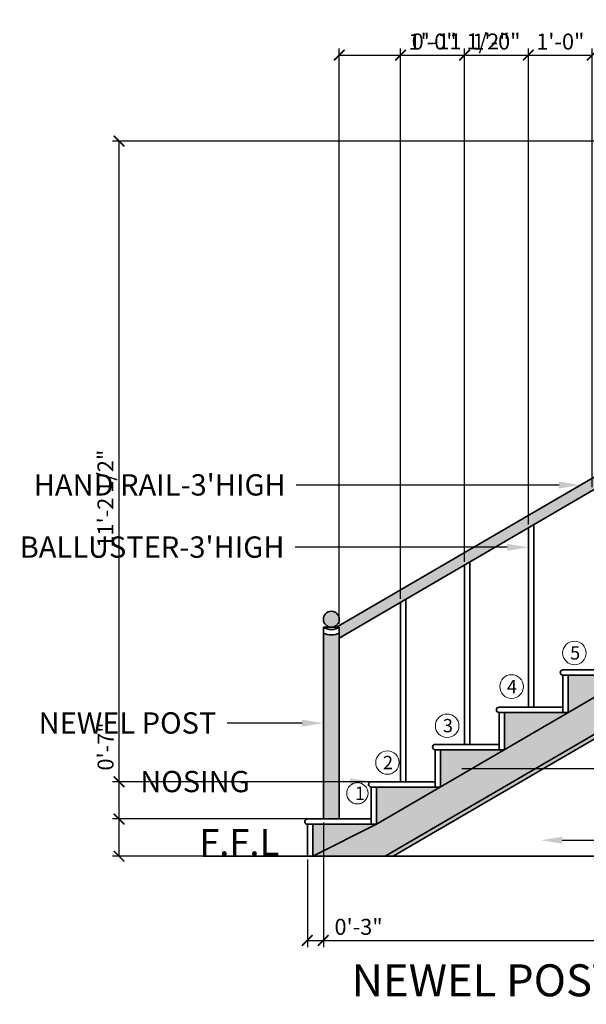
# Model space of a CAD drawing. Units: inches. Extents: x 2205 to 2524, y 4609 to 4803.
# Tile 1 of 5: x 2205 to 2311, y 4609 to 4794. Entities that reach past the tile are written whole.
import ezdxf
from ezdxf import colors
from ezdxf.entities.mleader import LeaderData, LeaderLine
from ezdxf.math import Vec2, Vec3

# ---------------------------------------------------------------- set-up
doc = ezdxf.new("R2010")
doc.units = ezdxf.units.IN
for name, color, linetype, lineweight in [('A-ANNO-DIMS', 2, 'Continuous', 18), ('A-ANNO-SYMB', 3, 'Continuous', 18), ('A-ANNO-TEXT', 7, 'Continuous', 18), ('A-FLOR-STRS', 7, 'Continuous', 35), ('A-SECT', 7, 'Continuous', 25), ('A-SECT-PATT', 252, 'Continuous', 13)]:
    doc.layers.add(name, color=color, linetype=linetype, lineweight=lineweight)
doc.styles.get("Standard").update_dxf_attribs({"font": 'arial.ttf'})
doc.dimstyles.new('ISO-25', dxfattribs={"dimtxt": 3, "dimasz": 2, "dimexe": 1.25, "dimexo": 0.625, "dimtad": 1, "dimdec": 1, "dimlunit": 3, "dimtxsty": 'Standard', "dimblk": 'ARCHTICK', "dimcen": 2.5, "dimclrd": 5, "dimclre": 2, "dimclrt": 6, "dimadec": 0, "dimazin": 0, "dimtfac": 1, "dimtdec": 1, "dimtmove": 0, "dimatfit": 3, "dimfxl": 1, "dimarcsym": 0})

# ---------------------------------------------------------------- blocks, each defined once
blk = doc.blocks.new('STAIR-STEP')
for p, q in [((2282.7, 4650.98), (2270.7, 4650.98)), ((2283.7, 4649.98), (2270.7, 4649.98)), ((2270.7, 4649.98), (2270.7, 4642.98)), ((2271.7, 4649.98), (2271.7, 4642.98))]:
    blk.add_line(p, q)
blk.add_arc((2270.7, 4650.48), 0.5, 90, 270)
blk = doc.blocks.new('NEWEL-POST')
for p, q in [((2261.7, 4679.98), (2261.7, 4643.98)), ((2261.71, 4679.98), (2261.7, 4679.98)), ((2261.71, 4679.98), (2264.69, 4679.98)), ((2264.7, 4679.98), (2264.69, 4679.98)), ((2264.7, 4679.98), (2264.7, 4643.98))]:
    blk.add_line(p, q)
blk.add_circle((2263.2, 4681.48), 1.5)
for radius, start, end in [(2.78, 237.6128, 302.3872), (3.78, 246.6124, 293.3876)]:
    blk.add_arc((2263.2, 4682.33), radius, start, end)
blk = doc.blocks.new('BALUSTER')
for p, q in [((2276.2, 4684.66), (2276.2, 4650.98)), ((2277.2, 4685.25), (2277.2, 4650.98))]:
    blk.add_line(p, q)
blk = doc.blocks.new('_ArchTick')
at = {"color": 0, "linetype": 'ByBlock', "const_width": 0.15}
blk.add_lwpolyline([(-0.5, -0.5), (0.5, 0.5)], dxfattribs=at)
blk = doc.blocks.new('*D15')
at = {"layer": 'A-ANNO-DIMS', "color": 2, "lineweight": -2, "transparency": 16777216}
for p, q in [((2258.7, 4636.35), (2258.7, 4619.93)), ((2429.2, 4636.35), (2429.2, 4619.93))]:
    blk.add_line(p, q, dxfattribs=at)
at = {"layer": 'A-ANNO-DIMS', "color": 5, "lineweight": -2, "transparency": 16777216}
blk.add_line((2258.7, 4621.18), (2429.2, 4621.18), dxfattribs=at)
at = {"layer": 'DEFPOINTS', "color": 0, "transparency": 16777216}
for p in [(2258.7, 4636.98), (2429.2, 4636.98), (2429.2, 4621.18)]:
    blk.add_point(p, dxfattribs=at)
at = {"layer": 'A-ANNO-DIMS', "color": 5, "lineweight": -2, "transparency": 16777216, "xscale": 2, "yscale": 2, "zscale": 2, "rotation": 180}
blk.add_blockref('_ArchTick', (2258.7, 4621.18), dxfattribs=at)
at = {"layer": 'A-ANNO-DIMS', "color": 5, "lineweight": -2, "transparency": 16777216, "xscale": 2, "yscale": 2, "zscale": 2}
blk.add_blockref('_ArchTick', (2429.2, 4621.18), dxfattribs=at)
at = {"layer": 'A-ANNO-DIMS', "color": 6, "transparency": 16777216, "insert": (2343.95, 4623.36), "char_height": 3, "attachment_point": 5}
blk.add_mtext('14\'-2 1/2"', dxfattribs=at)
blk = doc.blocks.new('*D16')
at = {"layer": 'A-ANNO-DIMS', "color": 2, "lineweight": -2, "transparency": 16777216}
for p, q in [((2428.57, 4771.26), (2222.09, 4771.26)), ((2428.57, 4636.98), (2222.09, 4636.98))]:
    blk.add_line(p, q, dxfattribs=at)
at = {"layer": 'A-ANNO-DIMS', "color": 5, "lineweight": -2, "transparency": 16777216}
blk.add_line((2223.34, 4636.98), (2223.34, 4771.26), dxfattribs=at)
at = {"layer": 'DEFPOINTS', "color": 0, "transparency": 16777216}
for p in [(2223.34, 4771.26), (2429.2, 4771.26), (2429.2, 4636.98)]:
    blk.add_point(p, dxfattribs=at)
at = {"layer": 'A-ANNO-DIMS', "color": 5, "lineweight": -2, "transparency": 16777216, "xscale": 2, "yscale": 2, "zscale": 2}
for p, rotation in [((2223.34, 4771.26), 90), ((2223.34, 4636.98), 270)]:
    blk.add_blockref('_ArchTick', p, dxfattribs=dict(at, rotation=rotation))
at = {"layer": 'A-ANNO-DIMS', "color": 6, "transparency": 16777216, "insert": (2221.17, 4704.12), "char_height": 3, "attachment_point": 5, "rotation": 90}
blk.add_mtext('11\'-2 1/2"', dxfattribs=at)
blk = doc.blocks.new('*D18')
at = {"layer": 'A-ANNO-DIMS', "color": 5, "lineweight": -2, "transparency": 16777216}
for p, q in [((2223.34, 4650.98), (2223.34, 4662.2)), ((2223.34, 4643.98), (2223.34, 4650.98))]:
    blk.add_line(p, q, dxfattribs=at)
at = {"layer": 'A-ANNO-DIMS', "color": 2, "lineweight": -2, "transparency": 16777216}
for p, q in [((2275.57, 4650.98), (2222.09, 4650.98)), ((2264.07, 4643.98), (2222.09, 4643.98))]:
    blk.add_line(p, q, dxfattribs=at)
at = {"layer": 'DEFPOINTS', "color": 0, "transparency": 16777216}
for p in [(2223.34, 4650.98), (2276.2, 4650.98), (2264.7, 4643.98)]:
    blk.add_point(p, dxfattribs=at)
at = {"layer": 'A-ANNO-DIMS', "color": 5, "lineweight": -2, "transparency": 16777216, "xscale": 2, "yscale": 2, "zscale": 2}
for p, rotation in [((2223.34, 4650.98), 90), ((2223.34, 4643.98), 270)]:
    blk.add_blockref('_ArchTick', p, dxfattribs=dict(at, rotation=rotation))
at = {"layer": 'A-ANNO-DIMS', "color": 6, "transparency": 16777216, "insert": (2221.19, 4657.59), "char_height": 3, "attachment_point": 5, "rotation": 90}
blk.add_mtext('0\'-7"', dxfattribs=at)
blk = doc.blocks.new('*D24')
at = {"layer": 'A-ANNO-DIMS', "color": 2, "lineweight": -2, "transparency": 16777216}
for p, q in [((2261.7, 4643.35), (2261.7, 4619.93)), ((2258.7, 4636.35), (2258.7, 4619.93))]:
    blk.add_line(p, q, dxfattribs=at)
at = {"layer": 'A-ANNO-DIMS', "color": 5, "lineweight": -2, "transparency": 16777216}
for p, q in [((2258.7, 4621.18), (2261.7, 4621.18)), ((2261.7, 4621.18), (2272.92, 4621.18))]:
    blk.add_line(p, q, dxfattribs=at)
at = {"layer": 'DEFPOINTS', "color": 0, "transparency": 16777216}
for p in [(2261.7, 4643.98), (2258.7, 4636.98), (2261.7, 4621.18)]:
    blk.add_point(p, dxfattribs=at)
at = {"layer": 'A-ANNO-DIMS', "color": 5, "lineweight": -2, "transparency": 16777216, "xscale": 2, "yscale": 2, "zscale": 2, "rotation": 180}
blk.add_blockref('_ArchTick', (2258.7, 4621.18), dxfattribs=at)
at = {"layer": 'A-ANNO-DIMS', "color": 5, "lineweight": -2, "transparency": 16777216, "xscale": 2, "yscale": 2, "zscale": 2}
blk.add_blockref('_ArchTick', (2261.7, 4621.18), dxfattribs=at)
at = {"layer": 'A-ANNO-DIMS', "color": 6, "transparency": 16777216, "insert": (2268.31, 4623.34), "char_height": 3, "attachment_point": 5}
blk.add_mtext('0\'-3"', dxfattribs=at)
blk = doc.blocks.new('*D26')
at = {"layer": 'A-ANNO-DIMS', "color": 2, "lineweight": -2, "transparency": 16777216}
for p, q in [((2264.7, 4680.6), (2264.7, 4788.66)), ((2276.2, 4685.29), (2276.2, 4788.66))]:
    blk.add_line(p, q, dxfattribs=at)
at = {"layer": 'A-ANNO-DIMS', "color": 5, "lineweight": -2, "transparency": 16777216}
for p, q in [((2264.7, 4787.41), (2276.2, 4787.41)), ((2276.2, 4787.41), (2296.74, 4787.41))]:
    blk.add_line(p, q, dxfattribs=at)
at = {"layer": 'DEFPOINTS', "color": 0, "transparency": 16777216}
for p in [(2276.2, 4787.41), (2276.2, 4684.66), (2264.7, 4679.98)]:
    blk.add_point(p, dxfattribs=at)
at = {"layer": 'A-ANNO-DIMS', "color": 5, "lineweight": -2, "transparency": 16777216, "xscale": 2, "yscale": 2, "zscale": 2, "rotation": 180}
blk.add_blockref('_ArchTick', (2264.7, 4787.41), dxfattribs=at)
at = {"layer": 'A-ANNO-DIMS', "color": 5, "lineweight": -2, "transparency": 16777216, "xscale": 2, "yscale": 2, "zscale": 2}
blk.add_blockref('_ArchTick', (2276.2, 4787.41), dxfattribs=at)
at = {"layer": 'A-ANNO-DIMS', "color": 6, "transparency": 16777216, "insert": (2287.47, 4789.58), "char_height": 3, "attachment_point": 5}
blk.add_mtext('0\'-11 1/2"', dxfattribs=at)
blk = doc.blocks.new('*D27')
at = {"layer": 'A-ANNO-DIMS', "color": 2, "lineweight": -2, "transparency": 16777216}
for p, q in [((2276.2, 4685.29), (2276.2, 4788.66)), ((2288.2, 4692.29), (2288.2, 4788.66))]:
    blk.add_line(p, q, dxfattribs=at)
at = {"layer": 'A-ANNO-DIMS', "color": 5, "lineweight": -2, "transparency": 16777216}
blk.add_line((2276.2, 4787.41), (2288.2, 4787.41), dxfattribs=at)
at = {"layer": 'DEFPOINTS', "color": 0, "transparency": 16777216}
for p in [(2288.2, 4787.41), (2288.2, 4691.66), (2276.2, 4684.66)]:
    blk.add_point(p, dxfattribs=at)
at = {"layer": 'A-ANNO-DIMS', "color": 5, "lineweight": -2, "transparency": 16777216, "xscale": 2, "yscale": 2, "zscale": 2, "rotation": 180}
blk.add_blockref('_ArchTick', (2276.2, 4787.41), dxfattribs=at)
at = {"layer": 'A-ANNO-DIMS', "color": 5, "lineweight": -2, "transparency": 16777216, "xscale": 2, "yscale": 2, "zscale": 2}
blk.add_blockref('_ArchTick', (2288.2, 4787.41), dxfattribs=at)
at = {"layer": 'A-ANNO-DIMS', "color": 6, "transparency": 16777216, "insert": (2282.2, 4789.56), "char_height": 3, "attachment_point": 5}
blk.add_mtext('1\'-0"', dxfattribs=at)
blk = doc.blocks.new('*D28')
at = {"layer": 'A-ANNO-DIMS', "color": 2, "lineweight": -2, "transparency": 16777216}
for p, q in [((2288.2, 4692.29), (2288.2, 4788.66)), ((2300.2, 4699.29), (2300.2, 4788.66))]:
    blk.add_line(p, q, dxfattribs=at)
at = {"layer": 'A-ANNO-DIMS', "color": 5, "lineweight": -2, "transparency": 16777216}
blk.add_line((2288.2, 4787.41), (2300.2, 4787.41), dxfattribs=at)
at = {"layer": 'DEFPOINTS', "color": 0, "transparency": 16777216}
for p in [(2300.2, 4787.41), (2300.2, 4698.66), (2288.2, 4691.66)]:
    blk.add_point(p, dxfattribs=at)
at = {"layer": 'A-ANNO-DIMS', "color": 5, "lineweight": -2, "transparency": 16777216, "xscale": 2, "yscale": 2, "zscale": 2, "rotation": 180}
blk.add_blockref('_ArchTick', (2288.2, 4787.41), dxfattribs=at)
at = {"layer": 'A-ANNO-DIMS', "color": 5, "lineweight": -2, "transparency": 16777216, "xscale": 2, "yscale": 2, "zscale": 2}
blk.add_blockref('_ArchTick', (2300.2, 4787.41), dxfattribs=at)
at = {"layer": 'A-ANNO-DIMS', "color": 6, "transparency": 16777216, "insert": (2294.2, 4789.56), "char_height": 3, "attachment_point": 5}
blk.add_mtext('1\'-0"', dxfattribs=at)
blk = doc.blocks.new('*D29')
at = {"layer": 'A-ANNO-DIMS', "color": 2, "lineweight": -2, "transparency": 16777216}
for p, q in [((2300.2, 4699.29), (2300.2, 4788.66)), ((2312.2, 4706.29), (2312.2, 4788.66))]:
    blk.add_line(p, q, dxfattribs=at)
at = {"layer": 'A-ANNO-DIMS', "color": 5, "lineweight": -2, "transparency": 16777216}
blk.add_line((2300.2, 4787.41), (2312.2, 4787.41), dxfattribs=at)
at = {"layer": 'DEFPOINTS', "color": 0, "transparency": 16777216}
for p in [(2312.2, 4787.41), (2312.2, 4705.66), (2300.2, 4698.66)]:
    blk.add_point(p, dxfattribs=at)
at = {"layer": 'A-ANNO-DIMS', "color": 5, "lineweight": -2, "transparency": 16777216, "xscale": 2, "yscale": 2, "zscale": 2, "rotation": 180}
blk.add_blockref('_ArchTick', (2300.2, 4787.41), dxfattribs=at)
at = {"layer": 'A-ANNO-DIMS', "color": 5, "lineweight": -2, "transparency": 16777216, "xscale": 2, "yscale": 2, "zscale": 2}
blk.add_blockref('_ArchTick', (2312.2, 4787.41), dxfattribs=at)
at = {"layer": 'A-ANNO-DIMS', "color": 6, "transparency": 16777216, "insert": (2306.2, 4789.56), "char_height": 3, "attachment_point": 5}
blk.add_mtext('1\'-0"', dxfattribs=at)

msp = doc.modelspace()

# ---------------------------------------------------------------- hatches: boundary and pattern name
at = {"layer": 'A-SECT-PATT'}
h = msp.add_hatch(dxfattribs=at)
h.set_pattern_fill('AR-CONC', color=256, scale=0.04)
h.paths.add_polyline_path([(2393.32, 4706.98), (2419.45, 4706.98), (2425.45, 4706.98), (2425.45, 4712.98), (2419.45, 4712.98), (2379.7, 4712.98), (2379.7, 4705.98), (2271.7, 4642.98), (2259.7, 4636.98), (2273.32, 4636.98)])
h.paths.add_polyline_path([(2343.7, 4684.98), (2331.7, 4684.98), (2331.7, 4677.98)], flags=16)
h.paths.add_polyline_path([(2331.7, 4677.98), (2319.7, 4677.98), (2319.7, 4670.98)], flags=16)
h.paths.add_polyline_path([(2319.7, 4670.98), (2307.7, 4670.98), (2307.7, 4663.98)], flags=16)
h.paths.add_polyline_path([(2307.7, 4663.98), (2295.7, 4663.98), (2295.7, 4656.98)], flags=16)
h.paths.add_polyline_path([(2295.7, 4656.98), (2283.7, 4656.98), (2283.7, 4649.98)], flags=16)
h.paths.add_polyline_path([(2283.7, 4649.98), (2271.7, 4649.98), (2271.7, 4642.98)], flags=17)
h.paths.add_polyline_path([(2271.7, 4642.98), (2259.7, 4642.98), (2259.7, 4636.98)], flags=17)
h.paths.add_polyline_path([(2379.7, 4705.98), (2367.7, 4705.98), (2367.7, 4698.98)], flags=16)
h.paths.add_polyline_path([(2367.7, 4698.98), (2355.7, 4698.98), (2355.7, 4691.98)], flags=16)
h.paths.add_polyline_path([(2419.45, 4706.98), (2393.32, 4706.98), (2273.32, 4636.98), (2274.81, 4636.98), (2393.52, 4706.23), (2419.45, 4706.23)], flags=17)
h.paths.add_polyline_path([(2419.45, 4706.23), (2418.7, 4706.23), (2418.7, 4636.98), (2419.45, 4636.98)], flags=16)
h.paths.add_polyline_path([(2429.2, 4771.26), (2428.45, 4771.26), (2428.45, 4636.98), (2429.2, 4636.98)])
h.paths.add_polyline_path([(2419.45, 4771.26), (2418.7, 4771.26), (2418.7, 4713.98), (2419.45, 4713.98)])
h = msp.add_hatch(color=256, dxfattribs=at)
h.dxf.hatch_style = 1
h.paths.add_polyline_path([(2264.7, 4678.86, -0.206977), (2261.7, 4678.86), (2261.7, 4643.98), (2264.7, 4643.98)])
h.paths.add_polyline_path([(2261.7, 4681.48, 1), (2264.7, 4681.48, 1)])
h.paths.add_polyline_path([(2382.06, 4746.42), (2382.06, 4748.73), (2264.2, 4679.98), (2264.69, 4679.98), (2264.7, 4679.98), (2264.7, 4677.96)])
h.paths.add_polyline_path([(2418.7, 4748.73), (2385.06, 4748.73), (2385.06, 4746.73), (2418.7, 4746.73)])
h.paths.add_polyline_path([(2385.06, 4748.86, -0.206977), (2382.06, 4748.86), (2382.06, 4713.98), (2385.06, 4713.98)])
h.paths.add_polyline_path([(2382.06, 4751.48, 1), (2385.06, 4751.48, 1)])

# ---------------------------------------------------------------- linework, layer by layer
at = {"layer": 'A-ANNO-SYMB'}
for centre, radius in [((2308.85, 4675.15), 2.21), ((2297.05, 4668.85), 2.22), ((2284.95, 4661.48), 2.21), ((2273.73, 4654.57), 2.2), ((2268.09, 4648.81), 2)]:
    msp.add_circle(centre, radius, dxfattribs=at)
at = {"layer": 'A-FLOR-STRS'}
for p, q in [((2264.2, 4679.98), (2382.06, 4748.73)), ((2264.7, 4677.96), (2382.06, 4746.42)), ((2273.32, 4636.98), (2393.32, 4706.98)), ((2271.7, 4642.98), (2379.7, 4705.98)), ((2274.81, 4636.98), (2393.52, 4706.23)), ((2270.7, 4643.98), (2258.7, 4643.98)), ((2271.7, 4642.98), (2258.7, 4642.98)), ((2258.7, 4642.98), (2258.7, 4636.98)), ((2259.7, 4642.98), (2259.7, 4636.98)), ((2271.7, 4642.98), (2259.7, 4636.98))]:
    msp.add_line(p, q, dxfattribs=at)
msp.add_arc((2258.7, 4643.48), 0.5, 90, 270, dxfattribs=at)
at = {"layer": 'A-SECT'}
msp.add_line((2239.14, 4636.98), (2429.2, 4636.98), dxfattribs=at)

# ---------------------------------------------------------------- block references
at = {"layer": 'A-FLOR-STRS'}
for name, p in [('BALUSTER', (24, 14)), ('BALUSTER', (12, 7)), ('BALUSTER', (0, 0)), ('NEWEL-POST', (0, 0)), ('STAIR-STEP', (36, 21)), ('STAIR-STEP', (24, 14)), ('STAIR-STEP', (12, 7)), ('STAIR-STEP', (0, 0))]:
    msp.add_blockref(name, p, dxfattribs=at)

# ---------------------------------------------------------------- texts
at = {"layer": 'A-ANNO-TEXT', "attachment_point": 1}
for s, width, heights, insert, char_height in [('5', 3.6522, [0], (2308.03, 4676.42), 2.5), ('4', 3.6522, [0], (2296.18, 4670.1), 2.5), ('3', 3.6522, [0], (2284.14, 4662.76), 2.5), ('2', 3.6522, [0], (2272.9, 4655.83), 2.5), ('1', 3.6522, [0], (2267.63, 4650.06), 2.5), ('F.F.L', 13.5213, [3.64], (2238.39, 4642.09), 5), ('{\\fArial|b1|i0|c0|p34;NEWEL POST QUATER TURN STAIR}', 215.8477, [0], (2266.99, 4616.69), 6)]:
    msp.add_mtext_dynamic_manual_height_columns(s, width=width, gutter_width=12.5, heights=heights, dxfattribs=dict(at, insert=insert, char_height=char_height))

# ---------------------------------------------------------------- dimensions: what is measured, and where the dimension line sits
at = {"layer": 'A-ANNO-DIMS'}
for base, p1, p2, picture, middle in [((2276.2, 4787.41), (2264.7, 4679.98), (2276.2, 4684.66), '*D26', (2287.47, 4789.58)), ((2288.2, 4787.41), (2276.2, 4684.66), (2288.2, 4691.66), '*D27', (2282.2, 4789.56)), ((2300.2, 4787.41), (2288.2, 4691.66), (2300.2, 4698.66), '*D28', (2294.2, 4789.56)), ((2312.2, 4787.41), (2300.2, 4698.66), (2312.2, 4705.66), '*D29', (2306.2, 4789.56)), ((2261.7, 4621.18), (2258.7, 4636.98), (2261.7, 4643.98), '*D24', (2268.31, 4623.34)), ((2429.2, 4621.18), (2258.7, 4636.98), (2429.2, 4636.98), '*D15', (2343.95, 4623.36))]:
    dim = msp.add_linear_dim(base=base, p1=p1, p2=p2, dimstyle='ISO-25', override={"dimdec": 1, "dimlfac": 1, "dimrnd": 0, "dimzin": 1, "dimdsep": 46, "dimlunit": 4, "dimfrac": 2}, dxfattribs=at)
    dim.commit()
    dim.dimension.update_dxf_attribs({"geometry": picture, "text_midpoint": middle})
for base, p1, p2, picture, middle in [((2223.34, 4771.26), (2429.2, 4636.98), (2429.2, 4771.26), '*D16', (2221.17, 4704.12)), ((2223.34, 4650.98), (2264.7, 4643.98), (2276.2, 4650.98), '*D18', (2221.19, 4657.59))]:
    dim = msp.add_linear_dim(base=base, p1=p1, p2=p2, angle=90, dimstyle='ISO-25', override={"dimdec": 1, "dimlfac": 1, "dimrnd": 0, "dimzin": 1, "dimdsep": 46, "dimlunit": 4, "dimfrac": 2}, dxfattribs=at)
    dim.commit()
    dim.dimension.update_dxf_attribs({"geometry": picture, "text_midpoint": middle})

# ---------------------------------------------------------------- leaders
at = {"layer": 'A-ANNO-SYMB'}
ml = msp.add_multileader_mtext('Standard', dxfattribs=at)
ml.set_content("HAND RAIL-3'HIGH", color=256)
ml.set_leader_properties()
ml.build(insert=Vec2(0, 0))
ctx = ml.context
ctx.base_point, ctx.plane_origin = Vec3(2203.7, 4706.67), Vec3(2309.96, 4706.67)
ctx.text_align_type = 2
notes = []
notes.append((ctx, [(0, (1, 1, 0), (2264.62, 4706.67), (-1, 0), 8, [(0, [(2309.96, 4706.67)], 0, [])])]))
ctx.mtext.insert, ctx.mtext.alignment, ctx.mtext.flow_direction = Vec3(2254.62, 4708.71), 3, 5
ml = msp.add_multileader_mtext('Standard', dxfattribs=at)
ml.set_content("BALLUSTER-3'HIGH", color=256)
ml.set_leader_properties()
ml.build(insert=Vec2(0, 0))
ctx = ml.context
ctx.base_point, ctx.plane_origin = Vec3(2200.63, 4694.99), Vec3(2300.2, 4694.99)
ctx.text_align_type = 2
notes.append((ctx, [(0, (1, 1, 0), (2264.39, 4694.99), (-1, 0), 8, [(0, [(2300.2, 4694.99)], 0, [])])]))
ctx.mtext.insert, ctx.mtext.alignment, ctx.mtext.flow_direction = Vec3(2254.39, 4697.03), 3, 5
ml = msp.add_multileader_mtext('Standard', dxfattribs=at)
ml.set_content('NEWEL POST', color=256)
ml.set_leader_properties()
ml.build(insert=Vec2(0, 0))
ctx = ml.context
ctx.base_point, ctx.plane_origin = Vec3(2203.51, 4661.98), Vec3(2261.7, 4661.98)
ctx.text_align_type = 2
notes.append((ctx, [(0, (1, 1, 0), (2251.61, 4661.98), (-1, 0), 8, [(0, [(2261.7, 4661.98)], 0, [])])]))
ctx.mtext.insert, ctx.mtext.alignment, ctx.mtext.flow_direction = Vec3(2241.61, 4664.01), 3, 5
ml = msp.add_multileader_mtext('Standard', dxfattribs=at)
ml.set_content('RISER', color=256)
ml.set_leader_properties()
ml.build(insert=Vec2(0, 0))
ctx = ml.context
ctx.base_point, ctx.plane_origin = Vec3(2321.78, 4653.48), Vec3(2283.7, 4653.48)
notes.append((ctx, [(0, (1, 1, 0), (2313.78, 4653.48), (1, 0), 8, [(0, [(2283.7, 4653.48)], 0, [])])]))
ctx.mtext.insert, ctx.mtext.width, ctx.mtext.flow_direction = Vec3(2323.78, 4655.51), 29.2708, 5
ml = msp.add_multileader_mtext('Standard', dxfattribs=at)
ml.set_content('NOSING', color=256)
ml.set_leader_properties()
ml.build(insert=Vec2(0, 0))
ctx = ml.context
ctx.base_point, ctx.plane_origin = Vec3(2224.61, 4650.98), Vec3(2270.7, 4650.98)
ctx.text_align_type = 2
notes.append((ctx, [(0, (1, 1, 0), (2257.87, 4650.98), (-1, 0), 8, [(0, [(2270.7, 4650.98)], 0, [])])]))
ctx.mtext.insert, ctx.mtext.alignment, ctx.mtext.flow_direction = Vec3(2247.87, 4653.01), 3, 5
ml = msp.add_multileader_mtext('Standard', dxfattribs=at)
ml.set_content('PITCH', color=256)
ml.set_leader_properties()
ml.build(insert=Vec2(0, 0))
ctx = ml.context
ctx.base_point, ctx.plane_origin = Vec3(2324.24, 4639.99), Vec3(2302.57, 4639.99)
notes.append((ctx, [(0, (1, 1, 0), (2316.24, 4639.99), (1, 0), 8, [(0, [(2302.57, 4639.99)], 0, [])])]))
ctx.mtext.insert, ctx.mtext.flow_direction = Vec3(2326.24, 4642.02), 5
for ctx, leaders in notes:
    for number, flags, end, landing, length, lines in leaders:
        leader = LeaderData()
        leader.index, (leader.has_last_leader_line, leader.has_dogleg_vector, leader.attachment_direction) = number, flags
        leader.last_leader_point, leader.dogleg_vector, leader.dogleg_length = Vec3(end), Vec3(landing), length
        for number, points, colour, breaks in lines:
            line = LeaderLine()
            line.index, line.vertices, line.color, line.breaks = number, Vec3.list(points), colors.encode_raw_color(colour), breaks
            leader.lines.append(line)
        ctx.leaders.append(leader)

doc.saveas('drawing.dxf')
